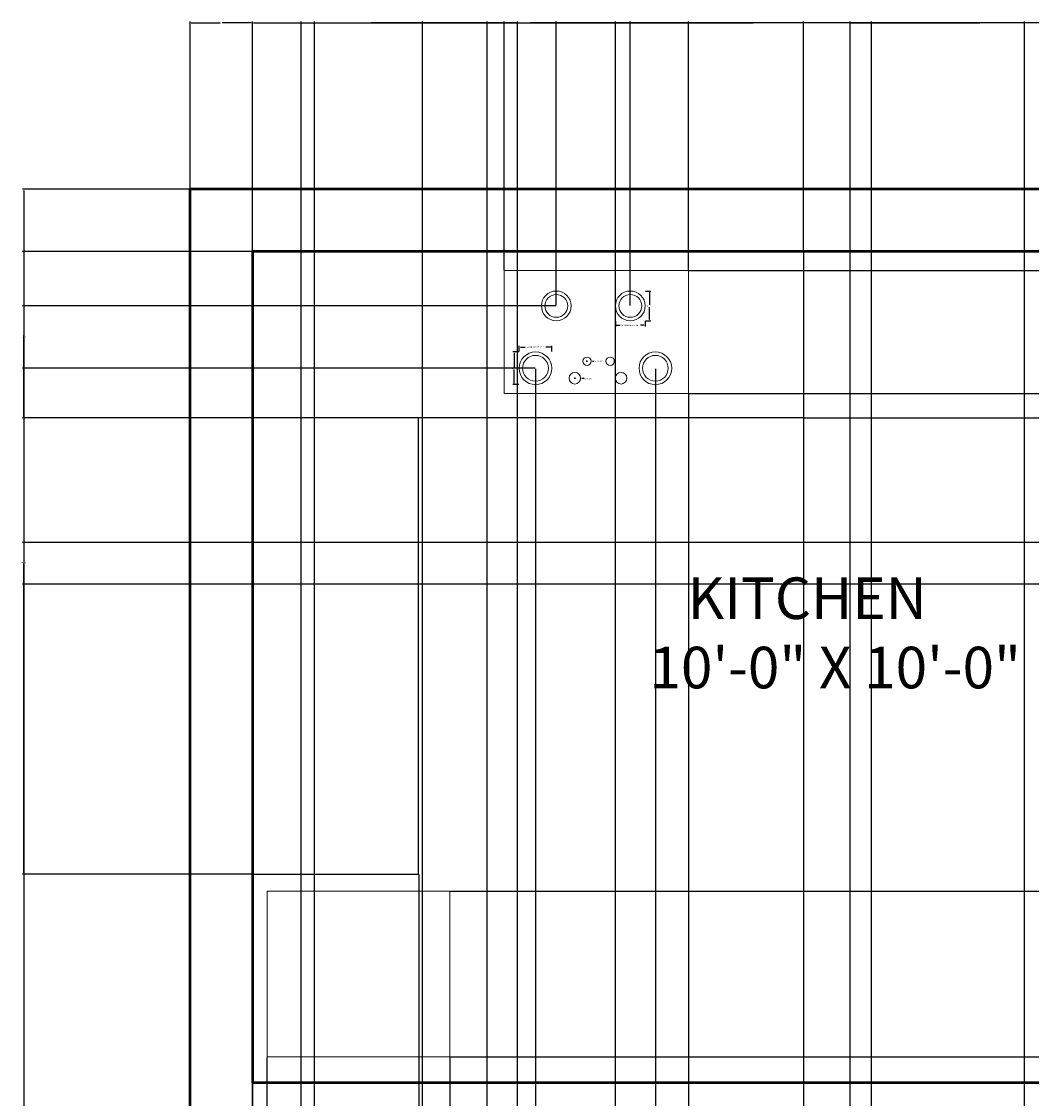
# Model space of a CAD drawing. Units: inches. Extents: x 2330 to 2739, y 947 to 1475.
# Tile 4 of 6: x 2330 to 2476, y 1320 to 1475. Entities that reach past the tile are written whole.
import ezdxf

# ---------------------------------------------------------------- set-up
doc = ezdxf.new("R2010")
doc.units = ezdxf.units.IN
for name, color, linetype, lineweight in [('A-ANNO-DIMS', 2, 'Continuous', 18), ('A-AREA-IDEN', 7, 'Continuous', 25), ('A-EQPM', 8, 'Continuous', 18), ('A-FLOR-FIXT', 9, 'Continuous', 25), ('wall', 7, 'Continuous', 50)]:
    doc.layers.add(name, color=color, linetype=linetype, lineweight=lineweight)
doc.styles.get("Standard").update_dxf_attribs({"font": 'arial.ttf'})
doc.dimstyles.get("Standard").update_dxf_attribs({"dimtxt": 0.18, "dimasz": 0.18, "dimexe": 0.18, "dimexo": 0.0625, "dimgap": 0.09, "dimtad": 0, "dimtih": 1, "dimtoh": 1, "dimdec": 4, "dimzin": 0, "dimdsep": 46, "dimtxsty": 'Standard', "dimcen": 0.09, "dimadec": 0, "dimazin": 0, "dimtfac": 1, "dimtdec": 4, "dimtofl": 0, "dimtmove": 0, "dimatfit": 3, "dimfxl": 1, "dimtolj": 1, "dimtzin": 0, "dimarcsym": 0})

# ---------------------------------------------------------------- blocks, each defined once
blk = doc.blocks.new('COOKTOP-BURNER-LARGE')
for radius in [2.36, 1.86]:
    blk.add_circle((0, 0), radius)
blk = doc.blocks.new('COOKTOP-BURNER-SMALL')
for radius in [2.15, 1.65]:
    blk.add_circle((0, 0), radius)
blk = doc.blocks.new('*D20')
at = {"layer": 'A-ANNO-DIMS', "color": 0, "lineweight": -2, "transparency": 16777216}
for p, q in [((2402.18, 1427.84), (2402.18, 1428.67)), ((2402.36, 1428.49), (2403.06, 1428.49)), ((2406.72, 1428.49), (2406.02, 1428.49)), ((2406.9, 1427.84), (2406.9, 1428.67))]:
    blk.add_line(p, q, dxfattribs=at)
at = {"layer": 'A-ANNO-DIMS', "color": 0, "transparency": 16777216}
for points in [[(2402.36, 1428.52), (2402.36, 1428.46), (2402.18, 1428.49)], [(2406.72, 1428.52), (2406.72, 1428.46), (2406.9, 1428.49)]]:
    blk.add_solid(points, dxfattribs=at)
at = {"layer": 'Defpoints', "color": 0, "transparency": 16777216}
for p in [(2406.9, 1428.49), (2402.18, 1427.78), (2406.9, 1427.78)]:
    blk.add_point(p, dxfattribs=at)
at = {"layer": 'A-ANNO-DIMS', "color": 0, "transparency": 16777216, "insert": (2404.54, 1428.49), "char_height": 0.18, "attachment_point": 5}
blk.add_mtext('\\A1;LARGE BURNER 5 TYP.', dxfattribs=at)
blk = doc.blocks.new('*D21')
at = {"layer": 'A-ANNO-DIMS', "color": 0, "lineweight": -2, "transparency": 16777216}
for p, q in [((2402.12, 1427.78), (2401.29, 1427.78)), ((2401.47, 1427.6), (2401.47, 1425.6)), ((2401.47, 1423.24), (2401.47, 1425.24)), ((2402.12, 1423.06), (2401.29, 1423.06))]:
    blk.add_line(p, q, dxfattribs=at)
at = {"layer": 'A-ANNO-DIMS', "color": 0, "transparency": 16777216}
for points in [[(2401.44, 1427.6), (2401.5, 1427.6), (2401.47, 1427.78)], [(2401.44, 1423.24), (2401.5, 1423.24), (2401.47, 1423.06)]]:
    blk.add_solid(points, dxfattribs=at)
at = {"layer": 'Defpoints', "color": 0, "transparency": 16777216}
for p in [(2401.47, 1427.78), (2402.18, 1427.78), (2402.18, 1423.06)]:
    blk.add_point(p, dxfattribs=at)
at = {"layer": 'A-ANNO-DIMS', "color": 0, "transparency": 16777216, "insert": (2401.47, 1425.42), "char_height": 0.18, "attachment_point": 5}
blk.add_mtext('\\A1;5 TYP.', dxfattribs=at)
blk = doc.blocks.new('*D22')
at = {"layer": 'A-ANNO-DIMS', "color": 0, "lineweight": -2, "transparency": 16777216}
for p, q in [((2416.07, 1432.21), (2416.07, 1431.45)), ((2416.25, 1431.63), (2416.75, 1431.63)), ((2420.19, 1431.63), (2419.69, 1431.63)), ((2420.37, 1432.21), (2420.37, 1431.45))]:
    blk.add_line(p, q, dxfattribs=at)
at = {"layer": 'A-ANNO-DIMS', "color": 0, "transparency": 16777216}
for points in [[(2416.25, 1431.66), (2416.25, 1431.6), (2416.07, 1431.63)], [(2420.19, 1431.66), (2420.19, 1431.6), (2420.37, 1431.63)]]:
    blk.add_solid(points, dxfattribs=at)
at = {"layer": 'Defpoints', "color": 0, "transparency": 16777216}
for p in [(2416.07, 1432.27), (2420.37, 1432.27), (2420.37, 1431.63)]:
    blk.add_point(p, dxfattribs=at)
at = {"layer": 'A-ANNO-DIMS', "color": 0, "transparency": 16777216, "insert": (2418.22, 1431.63), "char_height": 0.18, "attachment_point": 5}
blk.add_mtext('\\A1;SMALL BURNER 4 TYP.', dxfattribs=at)
blk = doc.blocks.new('*D23')
at = {"layer": 'A-ANNO-DIMS', "color": 0, "lineweight": -2, "transparency": 16777216}
for p, q in [((2420.43, 1436.57), (2421.19, 1436.57)), ((2421.01, 1436.39), (2421.01, 1434.6)), ((2421.01, 1432.45), (2421.01, 1434.24)), ((2420.43, 1432.27), (2421.19, 1432.27))]:
    blk.add_line(p, q, dxfattribs=at)
at = {"layer": 'A-ANNO-DIMS', "color": 0, "transparency": 16777216}
for points in [[(2420.98, 1436.39), (2421.04, 1436.39), (2421.01, 1436.57)], [(2420.98, 1432.45), (2421.04, 1432.45), (2421.01, 1432.27)]]:
    blk.add_solid(points, dxfattribs=at)
at = {"layer": 'Defpoints', "color": 0, "transparency": 16777216}
for p in [(2420.37, 1436.57), (2421.01, 1436.57), (2420.37, 1432.27)]:
    blk.add_point(p, dxfattribs=at)
at = {"layer": 'A-ANNO-DIMS', "color": 0, "transparency": 16777216, "insert": (2421.01, 1434.42), "char_height": 0.18, "attachment_point": 5}
blk.add_mtext('\\A1;4 TYP.', dxfattribs=at)
blk = doc.blocks.new('*D25')
at = {"layer": 'A-ANNO-DIMS', "color": 0, "lineweight": -2, "transparency": 16777216}
for p, q in [((2354.62, 1451.28), (2330.5, 1451.28)), ((2330.68, 1451.1), (2330.68, 1211.46)), ((2330.68, 971.46), (2330.68, 1211.1)), ((2354.62, 971.28), (2330.5, 971.28))]:
    blk.add_line(p, q, dxfattribs=at)
at = {"layer": 'A-ANNO-DIMS', "color": 0, "transparency": 16777216}
for points in [[(2330.65, 1451.1), (2330.71, 1451.1), (2330.68, 1451.28)], [(2330.65, 971.46), (2330.71, 971.46), (2330.68, 971.28)]]:
    blk.add_solid(points, dxfattribs=at)
at = {"layer": 'Defpoints', "color": 0, "transparency": 16777216}
for p in [(2330.68, 1451.28), (2354.68, 1451.28), (2354.68, 971.28)]:
    blk.add_point(p, dxfattribs=at)
at = {"layer": 'A-ANNO-DIMS', "color": 0, "transparency": 16777216, "insert": (2330.68, 1211.28), "char_height": 0.18, "attachment_point": 5}
blk.add_mtext('\\A1;480', dxfattribs=at)
blk = doc.blocks.new('*D33')
at = {"layer": 'A-ANNO-DIMS', "color": 0, "lineweight": -2, "transparency": 16777216}
for p, q in [((2363.68, 1130.34), (2363.68, 1475.46)), ((2363.86, 1475.28), (2382.41, 1475.28)), ((2401.75, 1475.28), (2383.2, 1475.28)), ((2401.93, 1130.34), (2401.93, 1475.46))]:
    blk.add_line(p, q, dxfattribs=at)
at = {"layer": 'A-ANNO-DIMS', "color": 0, "transparency": 16777216}
for points in [[(2363.86, 1475.31), (2363.86, 1475.25), (2363.68, 1475.28)], [(2401.75, 1475.31), (2401.75, 1475.25), (2401.93, 1475.28)]]:
    blk.add_solid(points, dxfattribs=at)
at = {"layer": 'Defpoints', "color": 0, "transparency": 16777216}
for p in [(2401.93, 1475.28), (2363.68, 1130.28), (2401.93, 1130.28)]:
    blk.add_point(p, dxfattribs=at)
at = {"layer": 'A-ANNO-DIMS', "color": 0, "transparency": 16777216, "insert": (2382.8, 1475.28), "char_height": 0.18, "attachment_point": 5}
blk.add_mtext('\\A1;38.25', dxfattribs=at)
blk = doc.blocks.new('*D34')
at = {"layer": 'A-ANNO-DIMS', "color": 0, "lineweight": -2, "transparency": 16777216}
for p, q in [((2449.93, 1139.34), (2449.93, 1475.46)), ((2450.11, 1475.28), (2468.66, 1475.28)), ((2488, 1475.28), (2469.45, 1475.28)), ((2488.18, 1139.34), (2488.18, 1475.46))]:
    blk.add_line(p, q, dxfattribs=at)
at = {"layer": 'A-ANNO-DIMS', "color": 0, "transparency": 16777216}
for points in [[(2450.11, 1475.31), (2450.11, 1475.25), (2449.93, 1475.28)], [(2488, 1475.31), (2488, 1475.25), (2488.18, 1475.28)]]:
    blk.add_solid(points, dxfattribs=at)
at = {"layer": 'Defpoints', "color": 0, "transparency": 16777216}
for p in [(2488.18, 1475.28), (2449.93, 1139.28), (2488.18, 1139.28)]:
    blk.add_point(p, dxfattribs=at)
at = {"layer": 'A-ANNO-DIMS', "color": 0, "transparency": 16777216, "insert": (2469.05, 1475.28), "char_height": 0.18, "attachment_point": 5}
blk.add_mtext('\\A1;38.25', dxfattribs=at)
blk = doc.blocks.new('*D44')
at = {"layer": 'A-ANNO-DIMS', "color": 0, "lineweight": -2, "transparency": 16777216}
for p, q in [((2370.71, 1254.55), (2370.71, 1475.46)), ((2370.89, 1475.28), (2383.67, 1475.28)), ((2397.37, 1475.28), (2384.6, 1475.28)), ((2397.55, 1254.55), (2397.55, 1475.46))]:
    blk.add_line(p, q, dxfattribs=at)
at = {"layer": 'A-ANNO-DIMS', "color": 0, "transparency": 16777216}
for points in [[(2370.89, 1475.31), (2370.89, 1475.25), (2370.71, 1475.28)], [(2397.37, 1475.31), (2397.37, 1475.25), (2397.55, 1475.28)]]:
    blk.add_solid(points, dxfattribs=at)
at = {"layer": 'Defpoints', "color": 0, "transparency": 16777216}
for p in [(2397.55, 1475.28), (2370.71, 1254.48), (2397.55, 1254.48)]:
    blk.add_point(p, dxfattribs=at)
at = {"layer": 'A-ANNO-DIMS', "color": 0, "transparency": 16777216, "insert": (2384.13, 1475.28), "char_height": 0.18, "attachment_point": 5}
blk.add_mtext('\\A1;26.846', dxfattribs=at)
blk = doc.blocks.new('*D46')
at = {"layer": 'A-ANNO-DIMS', "color": 0, "lineweight": -2, "transparency": 16777216}
for p, q in [((2416.07, 1232.48), (2416.07, 1475.46)), ((2416.25, 1475.28), (2434.16, 1475.28)), ((2452.86, 1475.28), (2434.95, 1475.28)), ((2453.04, 1232.48), (2453.04, 1475.46))]:
    blk.add_line(p, q, dxfattribs=at)
at = {"layer": 'A-ANNO-DIMS', "color": 0, "transparency": 16777216}
for points in [[(2416.25, 1475.31), (2416.25, 1475.25), (2416.07, 1475.28)], [(2452.86, 1475.31), (2452.86, 1475.25), (2453.04, 1475.28)]]:
    blk.add_solid(points, dxfattribs=at)
at = {"layer": 'Defpoints', "color": 0, "transparency": 16777216}
for p in [(2453.04, 1475.28), (2416.07, 1232.41), (2453.04, 1232.41)]:
    blk.add_point(p, dxfattribs=at)
at = {"layer": 'A-ANNO-DIMS', "color": 0, "transparency": 16777216, "insert": (2434.55, 1475.28), "char_height": 0.18, "attachment_point": 5}
blk.add_mtext('\\A1;36.97', dxfattribs=at)
blk = doc.blocks.new('*D48')
at = {"layer": 'A-ANNO-DIMS', "color": 0, "lineweight": -2, "transparency": 16777216}
for p, q in [((2397.55, 1177.11), (2397.55, 1475.46)), ((2397.73, 1475.28), (2435.93, 1475.28)), ((2474.92, 1475.28), (2436.72, 1475.28)), ((2475.1, 1177.11), (2475.1, 1475.46))]:
    blk.add_line(p, q, dxfattribs=at)
at = {"layer": 'A-ANNO-DIMS', "color": 0, "transparency": 16777216}
for points in [[(2397.73, 1475.31), (2397.73, 1475.25), (2397.55, 1475.28)], [(2474.92, 1475.31), (2474.92, 1475.25), (2475.1, 1475.28)]]:
    blk.add_solid(points, dxfattribs=at)
at = {"layer": 'Defpoints', "color": 0, "transparency": 16777216}
for p in [(2475.1, 1475.28), (2397.55, 1177.05), (2475.1, 1177.05)]:
    blk.add_point(p, dxfattribs=at)
at = {"layer": 'A-ANNO-DIMS', "color": 0, "transparency": 16777216, "insert": (2436.33, 1475.28), "char_height": 0.18, "attachment_point": 5}
blk.add_mtext('\\A1;77.54', dxfattribs=at)
blk = doc.blocks.new('*D50')
at = {"layer": 'A-ANNO-DIMS', "color": 0, "lineweight": -2, "transparency": 16777216}
for p, q in [((2372.63, 1173.51), (2372.63, 1475.46)), ((2372.81, 1475.28), (2379.98, 1475.28)), ((2388.05, 1475.28), (2380.88, 1475.28)), ((2388.23, 1173.51), (2388.23, 1475.46))]:
    blk.add_line(p, q, dxfattribs=at)
at = {"layer": 'A-ANNO-DIMS', "color": 0, "transparency": 16777216}
for points in [[(2372.81, 1475.31), (2372.81, 1475.25), (2372.63, 1475.28)], [(2388.05, 1475.31), (2388.05, 1475.25), (2388.23, 1475.28)]]:
    blk.add_solid(points, dxfattribs=at)
at = {"layer": 'Defpoints', "color": 0, "transparency": 16777216}
for p in [(2388.23, 1475.28), (2372.63, 1173.45), (2388.23, 1173.45)]:
    blk.add_point(p, dxfattribs=at)
at = {"layer": 'A-ANNO-DIMS', "color": 0, "transparency": 16777216, "insert": (2380.43, 1475.28), "char_height": 0.18, "attachment_point": 5}
blk.add_mtext('\\A1;15.592', dxfattribs=at)
blk = doc.blocks.new('*D56')
at = {"layer": 'A-ANNO-DIMS', "color": 0, "lineweight": -2, "transparency": 16777216}
for p, q in [((2354.68, 1451.34), (2354.68, 1475.46)), ((2354.86, 1475.28), (2359.03, 1475.28)), ((2363.5, 1475.28), (2359.33, 1475.28)), ((2363.68, 1442.34), (2363.68, 1475.46))]:
    blk.add_line(p, q, dxfattribs=at)
at = {"layer": 'A-ANNO-DIMS', "color": 0, "transparency": 16777216}
for points in [[(2354.86, 1475.31), (2354.86, 1475.25), (2354.68, 1475.28)], [(2363.5, 1475.31), (2363.5, 1475.25), (2363.68, 1475.28)]]:
    blk.add_solid(points, dxfattribs=at)
at = {"layer": 'Defpoints', "color": 0, "transparency": 16777216}
for p in [(2363.68, 1475.28), (2354.68, 1451.28), (2363.68, 1442.28)]:
    blk.add_point(p, dxfattribs=at)
at = {"layer": 'A-ANNO-DIMS', "color": 0, "transparency": 16777216, "insert": (2359.18, 1475.28), "char_height": 0.18, "attachment_point": 5}
blk.add_mtext('\\A1;9', dxfattribs=at)
blk = doc.blocks.new('*D57')
at = {"layer": 'A-ANNO-DIMS', "color": 0, "lineweight": -2, "transparency": 16777216}
for p, q in [((2363.68, 1442.34), (2363.68, 1475.46)), ((2363.86, 1475.28), (2403.05, 1475.28)), ((2443.02, 1475.28), (2403.83, 1475.28)), ((2443.2, 1442.34), (2443.2, 1475.46))]:
    blk.add_line(p, q, dxfattribs=at)
at = {"layer": 'A-ANNO-DIMS', "color": 0, "transparency": 16777216}
for points in [[(2363.86, 1475.31), (2363.86, 1475.25), (2363.68, 1475.28)], [(2443.02, 1475.31), (2443.02, 1475.25), (2443.2, 1475.28)]]:
    blk.add_solid(points, dxfattribs=at)
at = {"layer": 'Defpoints', "color": 0, "transparency": 16777216}
for p in [(2443.2, 1475.28), (2363.68, 1442.28), (2443.2, 1442.28)]:
    blk.add_point(p, dxfattribs=at)
at = {"layer": 'A-ANNO-DIMS', "color": 0, "transparency": 16777216, "insert": (2403.44, 1475.28), "char_height": 0.18, "attachment_point": 5}
blk.add_mtext('\\A1;79.52', dxfattribs=at)
blk = doc.blocks.new('*D58')
at = {"layer": 'A-ANNO-DIMS', "color": 0, "lineweight": -2, "transparency": 16777216}
for p, q in [((2363.62, 1442.28), (2330.5, 1442.28)), ((2330.68, 1442.1), (2330.68, 1397.53)), ((2330.68, 1352.6), (2330.68, 1397.17)), ((2363.62, 1352.42), (2330.5, 1352.42))]:
    blk.add_line(p, q, dxfattribs=at)
at = {"layer": 'A-ANNO-DIMS', "color": 0, "transparency": 16777216}
for points in [[(2330.65, 1442.1), (2330.71, 1442.1), (2330.68, 1442.28)], [(2330.65, 1352.6), (2330.71, 1352.6), (2330.68, 1352.42)]]:
    blk.add_solid(points, dxfattribs=at)
at = {"layer": 'Defpoints', "color": 0, "transparency": 16777216}
for p in [(2363.68, 1442.28), (2330.68, 1352.42), (2363.68, 1352.42)]:
    blk.add_point(p, dxfattribs=at)
at = {"layer": 'A-ANNO-DIMS', "color": 0, "transparency": 16777216, "insert": (2330.68, 1397.35), "char_height": 0.18, "attachment_point": 5}
blk.add_mtext('\\A1;89.86', dxfattribs=at)
blk = doc.blocks.new('*D59')
at = {"layer": 'A-ANNO-DIMS', "color": 0, "lineweight": -2, "transparency": 16777216}
for p, q in [((2363.68, 1352.36), (2363.68, 947.1)), ((2387.68, 1352.36), (2387.68, 947.1)), ((2363.86, 947.28), (2375.46, 947.28)), ((2387.5, 947.28), (2375.9, 947.28))]:
    blk.add_line(p, q, dxfattribs=at)
at = {"layer": 'A-ANNO-DIMS', "color": 0, "transparency": 16777216}
for points in [[(2363.86, 947.31), (2363.86, 947.25), (2363.68, 947.28)], [(2387.5, 947.31), (2387.5, 947.25), (2387.68, 947.28)]]:
    blk.add_solid(points, dxfattribs=at)
at = {"layer": 'Defpoints', "color": 0, "transparency": 16777216}
for p in [(2363.68, 1352.42), (2387.68, 1352.42), (2387.68, 947.28)]:
    blk.add_point(p, dxfattribs=at)
at = {"layer": 'A-ANNO-DIMS', "color": 0, "transparency": 16777216, "insert": (2375.68, 947.28), "char_height": 0.18, "attachment_point": 5}
blk.add_mtext('\\A1;24', dxfattribs=at)
blk = doc.blocks.new('*D60')
at = {"layer": 'A-ANNO-DIMS', "color": 0, "lineweight": -2, "transparency": 16777216}
for p, q in [((2443.13, 1442.28), (2330.5, 1442.28)), ((2330.68, 1442.1), (2330.68, 1430.46)), ((2330.68, 1418.46), (2330.68, 1430.1)), ((2443.13, 1418.28), (2330.5, 1418.28))]:
    blk.add_line(p, q, dxfattribs=at)
at = {"layer": 'A-ANNO-DIMS', "color": 0, "transparency": 16777216}
for points in [[(2330.65, 1442.1), (2330.71, 1442.1), (2330.68, 1442.28)], [(2330.65, 1418.46), (2330.71, 1418.46), (2330.68, 1418.28)]]:
    blk.add_solid(points, dxfattribs=at)
at = {"layer": 'Defpoints', "color": 0, "transparency": 16777216}
for p in [(2330.68, 1442.28), (2443.2, 1442.28), (2443.2, 1418.28)]:
    blk.add_point(p, dxfattribs=at)
at = {"layer": 'A-ANNO-DIMS', "color": 0, "transparency": 16777216, "insert": (2330.68, 1430.28), "char_height": 0.18, "attachment_point": 5}
blk.add_mtext('\\A1;24', dxfattribs=at)
blk = doc.blocks.new('*D61')
at = {"layer": 'A-ANNO-DIMS', "color": 0, "lineweight": -2, "transparency": 16777216}
for p, q in [((2400.02, 1439.6), (2400.02, 1475.46)), ((2400.2, 1475.28), (2412.94, 1475.28)), ((2426.46, 1475.28), (2413.73, 1475.28)), ((2426.64, 1439.6), (2426.64, 1475.46))]:
    blk.add_line(p, q, dxfattribs=at)
at = {"layer": 'A-ANNO-DIMS', "color": 0, "transparency": 16777216}
for points in [[(2400.2, 1475.31), (2400.2, 1475.25), (2400.02, 1475.28)], [(2426.46, 1475.31), (2426.46, 1475.25), (2426.64, 1475.28)]]:
    blk.add_solid(points, dxfattribs=at)
at = {"layer": 'Defpoints', "color": 0, "transparency": 16777216}
for p in [(2426.64, 1475.28), (2400.02, 1439.54), (2426.64, 1439.54)]:
    blk.add_point(p, dxfattribs=at)
at = {"layer": 'A-ANNO-DIMS', "color": 0, "transparency": 16777216, "insert": (2413.33, 1475.28), "char_height": 0.18, "attachment_point": 5}
blk.add_mtext('\\A1;26.62', dxfattribs=at)
blk = doc.blocks.new('*D62')
at = {"layer": 'A-ANNO-DIMS', "color": 0, "lineweight": -2, "transparency": 16777216}
for p, q in [((2426.7, 1439.54), (2738.86, 1439.54)), ((2738.68, 1439.36), (2738.68, 1430.83)), ((2738.68, 1421.95), (2738.68, 1430.47)), ((2426.7, 1421.77), (2738.86, 1421.77))]:
    blk.add_line(p, q, dxfattribs=at)
at = {"layer": 'A-ANNO-DIMS', "color": 0, "transparency": 16777216}
for points in [[(2738.65, 1439.36), (2738.71, 1439.36), (2738.68, 1439.54)], [(2738.65, 1421.95), (2738.71, 1421.95), (2738.68, 1421.77)]]:
    blk.add_solid(points, dxfattribs=at)
at = {"layer": 'Defpoints', "color": 0, "transparency": 16777216}
for p in [(2426.64, 1439.54), (2738.68, 1439.54), (2426.64, 1421.77)]:
    blk.add_point(p, dxfattribs=at)
at = {"layer": 'A-ANNO-DIMS', "color": 0, "transparency": 16777216, "insert": (2738.68, 1430.65), "char_height": 0.18, "attachment_point": 5}
blk.add_mtext('\\A1;17.77', dxfattribs=at)
blk = doc.blocks.new('*D63')
at = {"layer": 'A-ANNO-DIMS', "color": 0, "lineweight": -2, "transparency": 16777216}
for p, q in [((2426.64, 1421.71), (2426.64, 947.1)), ((2443.2, 1418.22), (2443.2, 947.1)), ((2426.82, 947.28), (2434.46, 947.28)), ((2443.02, 947.28), (2435.37, 947.28))]:
    blk.add_line(p, q, dxfattribs=at)
at = {"layer": 'A-ANNO-DIMS', "color": 0, "transparency": 16777216}
for points in [[(2426.82, 947.31), (2426.82, 947.25), (2426.64, 947.28)], [(2443.02, 947.31), (2443.02, 947.25), (2443.2, 947.28)]]:
    blk.add_solid(points, dxfattribs=at)
at = {"layer": 'Defpoints', "color": 0, "transparency": 16777216}
for p in [(2426.64, 1421.77), (2443.2, 1418.28), (2443.2, 947.28)]:
    blk.add_point(p, dxfattribs=at)
at = {"layer": 'A-ANNO-DIMS', "color": 0, "transparency": 16777216, "insert": (2434.92, 947.28), "char_height": 0.18, "attachment_point": 5}
blk.add_mtext('\\A1;16.556', dxfattribs=at)
blk = doc.blocks.new('*D64')
at = {"layer": 'A-ANNO-DIMS', "color": 0, "lineweight": -2, "transparency": 16777216}
for p, q in [((2426.7, 1421.77), (2738.86, 1421.77)), ((2738.68, 1421.59), (2738.68, 1420.21)), ((2738.68, 1418.46), (2738.68, 1419.84)), ((2443.26, 1418.28), (2738.86, 1418.28))]:
    blk.add_line(p, q, dxfattribs=at)
at = {"layer": 'A-ANNO-DIMS', "color": 0, "transparency": 16777216}
for points in [[(2738.65, 1421.59), (2738.71, 1421.59), (2738.68, 1421.77)], [(2738.65, 1418.46), (2738.71, 1418.46), (2738.68, 1418.28)]]:
    blk.add_solid(points, dxfattribs=at)
at = {"layer": 'Defpoints', "color": 0, "transparency": 16777216}
for p in [(2426.64, 1421.77), (2443.2, 1418.28), (2738.68, 1418.28)]:
    blk.add_point(p, dxfattribs=at)
at = {"layer": 'A-ANNO-DIMS', "color": 0, "transparency": 16777216, "insert": (2738.68, 1420.03), "char_height": 0.18, "attachment_point": 5}
blk.add_mtext('\\A1;3.487', dxfattribs=at)
blk = doc.blocks.new('*D65')
at = {"layer": 'A-ANNO-DIMS', "color": 0, "lineweight": -2, "transparency": 16777216}
for p, q in [((2404.54, 1425.36), (2404.54, 947.1)), ((2421.84, 1425.36), (2421.84, 947.1)), ((2404.72, 947.28), (2412.73, 947.28)), ((2421.66, 947.28), (2413.64, 947.28))]:
    blk.add_line(p, q, dxfattribs=at)
at = {"layer": 'A-ANNO-DIMS', "color": 0, "transparency": 16777216}
for points in [[(2404.72, 947.31), (2404.72, 947.25), (2404.54, 947.28)], [(2421.66, 947.31), (2421.66, 947.25), (2421.84, 947.28)]]:
    blk.add_solid(points, dxfattribs=at)
at = {"layer": 'Defpoints', "color": 0, "transparency": 16777216}
for p in [(2404.54, 1425.42), (2421.84, 1425.42), (2421.84, 947.28)]:
    blk.add_point(p, dxfattribs=at)
at = {"layer": 'A-ANNO-DIMS', "color": 0, "transparency": 16777216, "insert": (2413.19, 947.28), "char_height": 0.18, "attachment_point": 5}
blk.add_mtext('\\A1;17.295', dxfattribs=at)
blk = doc.blocks.new('*D66')
at = {"layer": 'A-ANNO-DIMS', "color": 0, "lineweight": -2, "transparency": 16777216}
for p, q in [((2407.54, 1434.48), (2407.54, 1475.46)), ((2407.72, 1475.28), (2412.49, 1475.28)), ((2418.04, 1475.28), (2413.26, 1475.28)), ((2418.22, 1434.48), (2418.22, 1475.46))]:
    blk.add_line(p, q, dxfattribs=at)
at = {"layer": 'A-ANNO-DIMS', "color": 0, "transparency": 16777216}
for points in [[(2407.72, 1475.31), (2407.72, 1475.25), (2407.54, 1475.28)], [(2418.04, 1475.31), (2418.04, 1475.25), (2418.22, 1475.28)]]:
    blk.add_solid(points, dxfattribs=at)
at = {"layer": 'Defpoints', "color": 0, "transparency": 16777216}
for p in [(2418.22, 1475.28), (2407.54, 1434.42), (2418.22, 1434.42)]:
    blk.add_point(p, dxfattribs=at)
at = {"layer": 'A-ANNO-DIMS', "color": 0, "transparency": 16777216, "insert": (2412.88, 1475.28), "char_height": 0.18, "attachment_point": 5}
blk.add_mtext('\\A1;10.68', dxfattribs=at)
blk = doc.blocks.new('*D67')
at = {"layer": 'A-ANNO-DIMS', "color": 0, "lineweight": -2, "transparency": 16777216}
for p, q in [((2407.47, 1434.42), (2330.5, 1434.42)), ((2330.68, 1434.24), (2330.68, 1430.1)), ((2330.68, 1425.6), (2330.68, 1429.74)), ((2404.48, 1425.42), (2330.5, 1425.42))]:
    blk.add_line(p, q, dxfattribs=at)
at = {"layer": 'A-ANNO-DIMS', "color": 0, "transparency": 16777216}
for points in [[(2330.65, 1434.24), (2330.71, 1434.24), (2330.68, 1434.42)], [(2330.65, 1425.6), (2330.71, 1425.6), (2330.68, 1425.42)]]:
    blk.add_solid(points, dxfattribs=at)
at = {"layer": 'Defpoints', "color": 0, "transparency": 16777216}
for p in [(2330.68, 1434.42), (2407.54, 1434.42), (2404.54, 1425.42)]:
    blk.add_point(p, dxfattribs=at)
at = {"layer": 'A-ANNO-DIMS', "color": 0, "transparency": 16777216, "insert": (2330.68, 1429.92), "char_height": 0.18, "attachment_point": 5}
blk.add_mtext('\\A1;9.003', dxfattribs=at)
blk = doc.blocks.new('*D70')
at = {"layer": 'A-ANNO-DIMS', "color": 0, "lineweight": -2, "transparency": 16777216}
for p, q in [((2365.79, 1325.96), (2365.79, 947.1)), ((2392.19, 1325.96), (2392.19, 947.1)), ((2365.97, 947.28), (2378.67, 947.28)), ((2392.01, 947.28), (2379.32, 947.28))]:
    blk.add_line(p, q, dxfattribs=at)
at = {"layer": 'A-ANNO-DIMS', "color": 0, "transparency": 16777216}
for points in [[(2365.97, 947.31), (2365.97, 947.25), (2365.79, 947.28)], [(2392.01, 947.31), (2392.01, 947.25), (2392.19, 947.28)]]:
    blk.add_solid(points, dxfattribs=at)
at = {"layer": 'Defpoints', "color": 0, "transparency": 16777216}
for p in [(2365.79, 1326.03), (2392.19, 1326.03), (2392.19, 947.28)]:
    blk.add_point(p, dxfattribs=at)
at = {"layer": 'A-ANNO-DIMS', "color": 0, "transparency": 16777216, "insert": (2378.99, 947.28), "char_height": 0.18, "attachment_point": 5}
blk.add_mtext('\\A1;26.4', dxfattribs=at)
blk = doc.blocks.new('*D71')
at = {"layer": 'A-ANNO-DIMS', "color": 0, "lineweight": -2, "transparency": 16777216}
for p, q in [((2392.26, 1349.96), (2738.86, 1349.96)), ((2738.68, 1349.78), (2738.68, 1338.17)), ((2738.68, 1326.21), (2738.68, 1337.81)), ((2392.26, 1326.03), (2738.86, 1326.03))]:
    blk.add_line(p, q, dxfattribs=at)
at = {"layer": 'A-ANNO-DIMS', "color": 0, "transparency": 16777216}
for points in [[(2738.65, 1349.78), (2738.71, 1349.78), (2738.68, 1349.96)], [(2738.65, 1326.21), (2738.71, 1326.21), (2738.68, 1326.03)]]:
    blk.add_solid(points, dxfattribs=at)
at = {"layer": 'Defpoints', "color": 0, "transparency": 16777216}
for p in [(2392.19, 1349.96), (2738.68, 1349.96), (2392.19, 1326.03)]:
    blk.add_point(p, dxfattribs=at)
at = {"layer": 'A-ANNO-DIMS', "color": 0, "transparency": 16777216, "insert": (2738.68, 1337.99), "char_height": 0.18, "attachment_point": 5}
blk.add_mtext('\\A1;23.93', dxfattribs=at)
blk = doc.blocks.new('*D79')
at = {"layer": 'A-ANNO-DIMS', "color": 0, "lineweight": -2, "transparency": 16777216}
for p, q in [((2608.12, 1400.28), (2330.5, 1400.28)), ((2330.68, 1400.1), (2330.68, 1397.46)), ((2330.68, 1394.46), (2330.68, 1397.1)), ((2608.12, 1394.28), (2330.5, 1394.28))]:
    blk.add_line(p, q, dxfattribs=at)
at = {"layer": 'A-ANNO-DIMS', "color": 0, "transparency": 16777216}
for points in [[(2330.65, 1400.1), (2330.71, 1400.1), (2330.68, 1400.28)], [(2330.65, 1394.46), (2330.71, 1394.46), (2330.68, 1394.28)]]:
    blk.add_solid(points, dxfattribs=at)
at = {"layer": 'Defpoints', "color": 0, "transparency": 16777216}
for p in [(2608.18, 1400.28), (2330.68, 1394.28), (2608.18, 1394.28)]:
    blk.add_point(p, dxfattribs=at)
at = {"layer": 'A-ANNO-DIMS', "color": 0, "transparency": 16777216, "insert": (2330.68, 1397.28), "char_height": 0.18, "attachment_point": 5}
blk.add_mtext('\\A1;6', dxfattribs=at)
blk = doc.blocks.new('*D84')
at = {"layer": 'A-ANNO-DIMS', "color": 0, "lineweight": -2, "transparency": 16777216}
for p, q in [((2411.88, 1426.44), (2412.06, 1426.44)), ((2411.97, 1426.35), (2411.97, 1426.53)), ((2412.94, 1426.41), (2412.75, 1426.42))]:
    blk.add_line(p, q, dxfattribs=at)
at = {"layer": 'A-ANNO-DIMS', "color": 0, "transparency": 16777216}
blk.add_solid([(2412.76, 1426.45), (2412.75, 1426.39), (2412.57, 1426.42)], dxfattribs=at)
at = {"layer": 'Defpoints', "color": 0, "transparency": 16777216}
for p in [(2411.37, 1426.46), (2412.57, 1426.42)]:
    blk.add_point(p, dxfattribs=at)
at = {"layer": 'A-ANNO-DIMS', "color": 0, "transparency": 16777216, "insert": (2413.62, 1426.41), "char_height": 0.18, "attachment_point": 5}
blk.add_mtext('\\A1;2X ∅1.205', dxfattribs=at)
blk = doc.blocks.new('*D85')
at = {"layer": 'A-ANNO-DIMS', "color": 0, "lineweight": -2, "transparency": 16777216}
for p, q in [((2410.12, 1423.98), (2410.3, 1423.98)), ((2410.21, 1423.89), (2410.21, 1424.07)), ((2411.54, 1423.93), (2411.22, 1423.95))]:
    blk.add_line(p, q, dxfattribs=at)
at = {"layer": 'A-ANNO-DIMS', "color": 0, "transparency": 16777216}
blk.add_solid([(2411.23, 1423.98), (2411.22, 1423.92), (2411.04, 1423.95)], dxfattribs=at)
at = {"layer": 'Defpoints', "color": 0, "transparency": 16777216}
for p in [(2409.38, 1424.01), (2411.04, 1423.95)]:
    blk.add_point(p, dxfattribs=at)
at = {"layer": 'A-ANNO-DIMS', "color": 0, "transparency": 16777216, "insert": (2412.16, 1423.93), "char_height": 0.18, "attachment_point": 5}
blk.add_mtext('\\A1;2X ∅1.67', dxfattribs=at)

msp = doc.modelspace()

# ---------------------------------------------------------------- linework, layer by layer
at = {"layer": 'A-EQPM'}
for points in [[(2400.0222, 1439.5396), (2426.6405, 1439.5396), (2426.6405, 1421.7694), (2400.0222, 1421.7694)], [(2392.1947, 1349.9582), (2365.7931, 1349.9582), (2365.7931, 1326.0264), (2392.1947, 1326.0264)]]:
    msp.add_lwpolyline(points, close=True, dxfattribs=at)
for centre, radius in [((2411.9723, 1426.4389), 0.6025), ((2415.3117, 1426.4389), 0.6025), ((2410.2098, 1423.9828), 0.8349), ((2416.8887, 1423.9828), 0.8349)]:
    msp.add_circle(centre, radius, dxfattribs=at)
at = {"layer": 'A-FLOR-FIXT'}
for p, q in [((2443.1961, 1442.2823), (2443.1961, 1418.2823)), ((2443.1961, 1418.2823), (2387.6781, 1418.2823)), ((2387.6781, 1352.4216), (2387.6781, 1418.2823)), ((2363.6781, 1352.4216), (2387.6781, 1352.4216))]:
    msp.add_line(p, q, dxfattribs=at)
at = {"layer": 'wall'}
for p, q in [((2714.6781, 1451.2823), (2354.6781, 1451.2823)), ((2354.6781, 1451.2823), (2354.6781, 971.2823)), ((2363.6781, 1442.2823), (2363.6781, 1322.2823)), ((2483.6781, 1442.2823), (2363.6781, 1442.2823)), ((2483.6781, 1322.2823), (2363.6781, 1322.2823))]:
    msp.add_line(p, q, dxfattribs=at)

# ---------------------------------------------------------------- block references
at = {"layer": 'A-EQPM'}
for name, p in [('COOKTOP-BURNER-SMALL', (2407.5363, 1434.4225)), ('COOKTOP-BURNER-SMALL', (2418.2173, 1434.4225)), ('COOKTOP-BURNER-LARGE', (2404.5411, 1425.4192)), ('COOKTOP-BURNER-LARGE', (2421.8362, 1425.4192))]:
    msp.add_blockref(name, p, dxfattribs=at)

# ---------------------------------------------------------------- texts
at = {"layer": 'A-AREA-IDEN', "insert": (2420.9844, 1395.2294), "char_height": 6, "attachment_point": 1}
msp.add_mtext_dynamic_manual_height_columns('   KITCHEN\\P10\'-0" X 10\'-0"', width=63.218259, gutter_width=12.5, heights=[0], dxfattribs=at)

# ---------------------------------------------------------------- dimensions: what is measured, and where the dimension line sits
at = {"layer": 'A-ANNO-DIMS'}
for base, p1, p2, override, picture, middle in [((2363.6781, 1475.2843), (2354.6781, 1451.2823), (2363.6781, 1442.2823), {"dimdec": 0, "dimlfac": 1, "dimrnd": 0, "dimzin": 0, "dimdsep": 46, "dimlunit": 2}, '*D56', (2359.1781, 1475.2843)), ((2401.9281, 1475.2843), (2363.6781, 1130.2823), (2401.9281, 1130.2823), {"dimdec": 2, "dimlfac": 1, "dimrnd": 0, "dimzin": 0, "dimdsep": 46, "dimlunit": 2}, '*D33', (2382.8031, 1475.2843)), ((2443.1961, 1475.2843), (2363.6781, 1442.2823), (2443.1961, 1442.2823), {"dimdec": 2, "dimlfac": 1, "dimrnd": 0, "dimzin": 0, "dimdsep": 46, "dimlunit": 2}, '*D57', (2403.4371, 1475.2843)), ((2397.5542, 1475.2843), (2370.708, 1254.4842), (2397.5542, 1254.4842), {"dimdec": 3, "dimlfac": 1, "dimrnd": 0, "dimzin": 0, "dimdsep": 46, "dimlunit": 2}, '*D44', (2384.1311, 1475.2843)), ((2388.2258, 1475.2843), (2372.634, 1173.4475), (2388.2258, 1173.4475), {"dimdec": 3, "dimlfac": 1, "dimrnd": 0, "dimzin": 0, "dimdsep": 46, "dimlunit": 2}, '*D50', (2380.4299, 1475.2843)), ((2475.0968, 1475.2843), (2397.5542, 1177.0487), (2475.0968, 1177.0487), {"dimdec": 2, "dimlfac": 1, "dimrnd": 0, "dimzin": 0, "dimdsep": 46, "dimlunit": 2}, '*D48', (2436.3255, 1475.2843)), ((2426.6405, 1475.2843), (2400.0222, 1439.5396), (2426.6405, 1439.5396), {"dimdec": 2, "dimlfac": 1, "dimrnd": 0, "dimzin": 0, "dimdsep": 46, "dimlunit": 2}, '*D61', (2413.3314, 1475.2843)), ((2418.2173, 1475.2843), (2407.5363, 1434.4225), (2418.2173, 1434.4225), {"dimdec": 2, "dimlfac": 1, "dimrnd": 0, "dimzin": 0, "dimdsep": 46, "dimlunit": 2}, '*D66', (2412.8768, 1475.2843)), ((2453.0384, 1475.2843), (2416.0685, 1232.4146), (2453.0384, 1232.4146), {"dimdec": 2, "dimlfac": 1, "dimrnd": 0, "dimzin": 0, "dimdsep": 46, "dimlunit": 2}, '*D46', (2434.5534, 1475.2843)), ((2488.1781, 1475.2843), (2449.9281, 1139.2823), (2488.1781, 1139.2823), {"dimdec": 2, "dimlfac": 1, "dimrnd": 0, "dimzin": 0, "dimdsep": 46, "dimlunit": 2}, '*D34', (2469.0531, 1475.2843)), ((2421.8362, 947.2803), (2404.5411, 1425.4192), (2421.8362, 1425.4192), {"dimdec": 3, "dimlfac": 1, "dimrnd": 0, "dimzin": 0, "dimdsep": 46, "dimlunit": 2}, '*D65', (2413.1887, 947.2803)), ((2443.1961, 947.2803), (2426.6405, 1421.7694), (2443.1961, 1418.2823), {"dimdec": 3, "dimlfac": 1, "dimrnd": 0, "dimzin": 0, "dimdsep": 46, "dimlunit": 2}, '*D63', (2434.9183, 947.2803)), ((2387.6781, 947.2803), (2363.6781, 1352.4216), (2387.6781, 1352.4216), {"dimdec": 0, "dimlfac": 1, "dimrnd": 0, "dimzin": 0, "dimdsep": 46, "dimlunit": 2}, '*D59', (2375.6781, 947.2803)), ((2392.1947, 947.2803), (2365.7931, 1326.0264), (2392.1947, 1326.0264), {"dimdec": 1, "dimlfac": 1, "dimrnd": 0, "dimzin": 0, "dimdsep": 46, "dimlunit": 2}, '*D70', (2378.9939, 947.2803))]:
    dim = msp.add_linear_dim(base=base, p1=p1, p2=p2, dimstyle='Standard', override=override, dxfattribs=at)
    dim.commit()
    dim.dimension.update_dxf_attribs({"geometry": picture, "text_midpoint": middle})
for base, p1, p2, override, picture, middle in [((2330.6761, 1451.2823), (2354.6781, 971.2823), (2354.6781, 1451.2823), {"dimdec": 0, "dimlfac": 1, "dimrnd": 0, "dimzin": 0, "dimdsep": 46, "dimlunit": 2}, '*D25', (2330.6761, 1211.2823)), ((2330.6761, 1352.4216), (2363.6781, 1442.2823), (2363.6781, 1352.4216), {"dimdec": 2, "dimlfac": 1, "dimrnd": 0, "dimzin": 0, "dimdsep": 46, "dimlunit": 2}, '*D58', (2330.6761, 1397.3519)), ((2330.6761, 1442.2823), (2443.1961, 1418.2823), (2443.1961, 1442.2823), {"dimdec": 0, "dimlfac": 1, "dimrnd": 0, "dimzin": 0, "dimdsep": 46, "dimlunit": 2}, '*D60', (2330.6761, 1430.2823)), ((2738.6801, 1439.5396), (2426.6405, 1421.7694), (2426.6405, 1439.5396), {"dimdec": 2, "dimlfac": 1, "dimrnd": 0, "dimzin": 0, "dimdsep": 46, "dimlunit": 2}, '*D62', (2738.6801, 1430.6545)), ((2330.6761, 1434.4225), (2404.5411, 1425.4192), (2407.5363, 1434.4225), {"dimdec": 3, "dimlfac": 1, "dimrnd": 0, "dimzin": 0, "dimdsep": 46, "dimlunit": 2}, '*D67', (2330.6761, 1429.9208)), ((2738.6801, 1418.2823), (2426.6405, 1421.7694), (2443.1961, 1418.2823), {"dimdec": 3, "dimlfac": 1, "dimrnd": 0, "dimzin": 0, "dimdsep": 46, "dimlunit": 2}, '*D64', (2738.6801, 1420.0258)), ((2330.6761, 1394.2823), (2608.1781, 1400.2823), (2608.1781, 1394.2823), {"dimdec": 0, "dimlfac": 1, "dimrnd": 0, "dimzin": 0, "dimdsep": 46, "dimlunit": 2}, '*D79', (2330.6761, 1397.2823)), ((2738.6801, 1349.9582), (2392.1947, 1326.0264), (2392.1947, 1349.9582), {"dimdec": 2, "dimlfac": 1, "dimrnd": 0, "dimzin": 0, "dimdsep": 46, "dimlunit": 2}, '*D71', (2738.6801, 1337.9923))]:
    dim = msp.add_linear_dim(base=base, p1=p1, p2=p2, angle=90, dimstyle='Standard', override=override, dxfattribs=at)
    dim.commit()
    dim.dimension.update_dxf_attribs({"geometry": picture, "text_midpoint": middle})
for base, p1, p2, picture, middle in [((2421.0118, 1436.5721), (2420.3669, 1432.2729), (2420.3669, 1436.5721), '*D23', (2421.0118, 1434.4225)), ((2401.469, 1427.7824), (2402.1779, 1423.056), (2402.1779, 1427.7824), '*D21', (2401.469, 1425.4192))]:
    dim = msp.add_linear_dim(base=base, p1=p1, p2=p2, angle=90, text='<> TYP.', dimstyle='Standard', override={"dimdec": 0, "dimlfac": 1, "dimrnd": 0, "dimzin": 0, "dimdsep": 46, "dimlunit": 2}, dxfattribs=at)
    dim.commit()
    dim.dimension.update_dxf_attribs({"geometry": picture, "text_midpoint": middle})
for base, p1, p2, text, picture, middle in [((2420.3669, 1431.628), (2416.0677, 1432.2729), (2420.3669, 1432.2729), 'SMALL BURNER <> TYP.', '*D22', (2418.2173, 1431.628)), ((2406.9043, 1428.4913), (2402.1779, 1427.7824), (2406.9043, 1427.7824), 'LARGE BURNER <> TYP.', '*D20', (2404.5411, 1428.4913))]:
    dim = msp.add_linear_dim(base=base, p1=p1, p2=p2, text=text, dimstyle='Standard', override={"dimdec": 0, "dimlfac": 1, "dimrnd": 0, "dimzin": 0, "dimdsep": 46, "dimlunit": 2}, dxfattribs=at)
    dim.commit()
    dim.dimension.update_dxf_attribs({"geometry": picture, "text_midpoint": middle})
for p1, p2, override, picture, middle in [((2411.3701, 1426.4571), (2412.5744, 1426.4208), {"dimdec": 3, "dimlfac": 1, "dimrnd": 0, "dimzin": 0, "dimdsep": 46, "dimlunit": 2}, '*D84', (2412.9357, 1426.4099)), ((2409.3755, 1424.0131), (2411.0441, 1423.9524), {"dimdec": 2, "dimlfac": 1, "dimrnd": 0, "dimzin": 0, "dimdsep": 46, "dimlunit": 2}, '*D85', (2411.5447, 1423.9342))]:
    dim = msp.add_diameter_dim_2p(p1=p1, p2=p2, text='2X <>', dimstyle='Standard', override=override, dxfattribs=at)
    dim.commit()
    dim.dimension.update_dxf_attribs({"geometry": picture, "text_midpoint": middle, "dimtype": 163})

doc.saveas('drawing.dxf')
